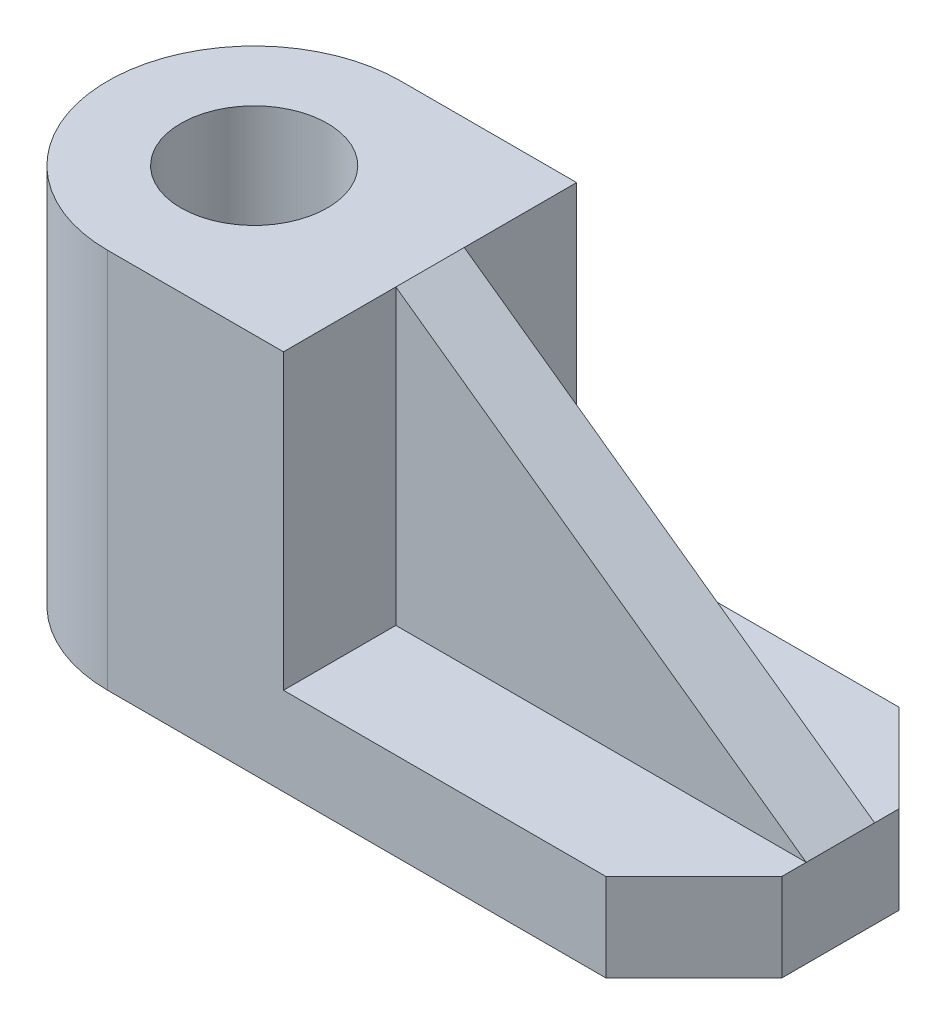
ISO-10303-21;
HEADER;
FILE_DESCRIPTION(('STEP AP214'),'2;1');
FILE_NAME('part.step','',(''),(''),'','','');
FILE_SCHEMA(('AUTOMOTIVE_DESIGN { 1 0 10303 214 1 1 1 1 }'));
ENDSEC;
DATA;
#1=APPLICATION_CONTEXT('core data for automotive mechanical design processes');
#2=APPLICATION_PROTOCOL_DEFINITION('international standard','automotive_design',2000,#1);
#3=PRODUCT_CONTEXT('',#1,'mechanical');
#4=PRODUCT('Part','Part','',(#3));
#5=PRODUCT_RELATED_PRODUCT_CATEGORY('part','',(#4));
#6=PRODUCT_DEFINITION_FORMATION('','',#4);
#7=PRODUCT_DEFINITION_CONTEXT('part definition',#1,'design');
#8=PRODUCT_DEFINITION('design','',#6,#7);
#9=PRODUCT_DEFINITION_SHAPE('','',#8);
#10=(LENGTH_UNIT() NAMED_UNIT(*) SI_UNIT(.MILLI.,.METRE.));
#11=(NAMED_UNIT(*) PLANE_ANGLE_UNIT() SI_UNIT($,.RADIAN.));
#12=(NAMED_UNIT(*) SI_UNIT($,.STERADIAN.) SOLID_ANGLE_UNIT());
#13=UNCERTAINTY_MEASURE_WITH_UNIT(LENGTH_MEASURE(1.E-05),#10,'distance_accuracy_value','');
#14=(GEOMETRIC_REPRESENTATION_CONTEXT(3) GLOBAL_UNCERTAINTY_ASSIGNED_CONTEXT((#13)) GLOBAL_UNIT_ASSIGNED_CONTEXT((#10,
#11,#12)) REPRESENTATION_CONTEXT('',''));
#15=CARTESIAN_POINT('',(0.,0.,0.));
#16=DIRECTION('',(0.,0.,1.));
#17=DIRECTION('',(1.,0.,0.));
#18=AXIS2_PLACEMENT_3D('',#15,#16,#17);
#19=CARTESIAN_POINT('',(0.,9.,0.));
#20=DIRECTION('',(0.,1.,0.));
#21=DIRECTION('',(0.,0.,1.));
#22=AXIS2_PLACEMENT_3D('',#19,#20,#21);
#23=PLANE('',#22);
#24=DIRECTION('',(0.,0.,1.));
#25=VECTOR('',#24,1.);
#26=CARTESIAN_POINT('',(-4.5,9.,0.));
#27=LINE('',#26,#25);
#28=CARTESIAN_POINT('',(-4.5,9.,-15.));
#29=VERTEX_POINT('',#28);
#30=CARTESIAN_POINT('',(-4.5,9.,-3.5));
#31=VERTEX_POINT('',#30);
#32=EDGE_CURVE('E166',#29,#31,#27,.T.);
#33=ORIENTED_EDGE('',*,*,#32,.T.);
#34=DIRECTION('',(1.,0.,0.));
#35=VECTOR('',#34,1.);
#36=CARTESIAN_POINT('',(37.5,9.,-3.5));
#37=LINE('',#36,#35);
#38=CARTESIAN_POINT('',(37.5,9.,-3.5));
#39=VERTEX_POINT('',#38);
#40=EDGE_CURVE('E59',#31,#39,#37,.T.);
#41=ORIENTED_EDGE('',*,*,#40,.T.);
#42=DIRECTION('',(0.,0.,-1.));
#43=VECTOR('',#42,1.);
#44=CARTESIAN_POINT('',(37.5,9.,-6.));
#45=LINE('',#44,#43);
#46=CARTESIAN_POINT('',(37.5,9.,-6.));
#47=VERTEX_POINT('',#46);
#48=EDGE_CURVE('E194',#39,#47,#45,.T.);
#49=ORIENTED_EDGE('',*,*,#48,.T.);
#50=DIRECTION('',(-0.707106781186548,0.,-0.707106781186547));
#51=VECTOR('',#50,1.);
#52=CARTESIAN_POINT('',(28.5,9.,-15.));
#53=LINE('',#52,#51);
#54=CARTESIAN_POINT('',(28.5,9.,-15.));
#55=VERTEX_POINT('',#54);
#56=EDGE_CURVE('E197',#47,#55,#53,.T.);
#57=ORIENTED_EDGE('',*,*,#56,.T.);
#58=DIRECTION('',(-1.,0.,0.));
#59=VECTOR('',#58,1.);
#60=CARTESIAN_POINT('',(-37.5,9.,-15.));
#61=LINE('',#60,#59);
#62=EDGE_CURVE('E200',#55,#29,#61,.T.);
#63=ORIENTED_EDGE('',*,*,#62,.T.);
#64=EDGE_LOOP('',(#33,#41,#49,#57,#63));
#65=FACE_BOUND('',#64,.T.);
#66=ADVANCED_FACE('F43',(#65),#23,.T.);
#67=CARTESIAN_POINT('',(-4.5,39.,0.));
#68=DIRECTION('',(1.,0.,0.));
#69=DIRECTION('',(0.,0.,-1.));
#70=AXIS2_PLACEMENT_3D('',#67,#68,#69);
#71=PLANE('',#70);
#72=DIRECTION('',(0.,0.,1.));
#73=VECTOR('',#72,1.);
#74=CARTESIAN_POINT('',(-4.5,39.,0.));
#75=LINE('',#74,#73);
#76=CARTESIAN_POINT('',(-4.5,39.,-15.));
#77=VERTEX_POINT('',#76);
#78=CARTESIAN_POINT('',(-4.5,39.,-3.5));
#79=VERTEX_POINT('',#78);
#80=EDGE_CURVE('E137',#77,#79,#75,.T.);
#81=ORIENTED_EDGE('',*,*,#80,.T.);
#82=DIRECTION('',(0.,-1.,0.));
#83=VECTOR('',#82,1.);
#84=CARTESIAN_POINT('',(-4.5,9.,-3.5));
#85=LINE('',#84,#83);
#86=EDGE_CURVE('E238',#79,#31,#85,.T.);
#87=ORIENTED_EDGE('',*,*,#86,.T.);
#88=ORIENTED_EDGE('',*,*,#32,.F.);
#89=DIRECTION('',(0.,-1.,0.));
#90=VECTOR('',#89,1.);
#91=CARTESIAN_POINT('',(-4.5,39.,-15.));
#92=LINE('',#91,#90);
#93=EDGE_CURVE('E177',#77,#29,#92,.T.);
#94=ORIENTED_EDGE('',*,*,#93,.F.);
#95=EDGE_LOOP('',(#81,#87,#88,#94));
#96=FACE_BOUND('',#95,.T.);
#97=ADVANCED_FACE('F265',(#96),#71,.T.);
#98=DIRECTION('',(1.,0.,0.));
#99=VECTOR('',#98,1.);
#100=CARTESIAN_POINT('',(37.5,9.,3.5));
#101=LINE('',#100,#99);
#102=CARTESIAN_POINT('',(-4.5,9.,3.5));
#103=VERTEX_POINT('',#102);
#104=CARTESIAN_POINT('',(37.5,9.,3.5));
#105=VERTEX_POINT('',#104);
#106=EDGE_CURVE('E151',#103,#105,#101,.T.);
#107=ORIENTED_EDGE('',*,*,#106,.F.);
#108=CARTESIAN_POINT('',(-4.5,9.,15.));
#109=VERTEX_POINT('',#108);
#110=EDGE_CURVE('E146',#103,#109,#27,.T.);
#111=ORIENTED_EDGE('',*,*,#110,.T.);
#112=DIRECTION('',(1.,0.,0.));
#113=VECTOR('',#112,1.);
#114=CARTESIAN_POINT('',(-37.5,9.,15.));
#115=LINE('',#114,#113);
#116=CARTESIAN_POINT('',(28.5,9.,15.));
#117=VERTEX_POINT('',#116);
#118=EDGE_CURVE('E186',#109,#117,#115,.T.);
#119=ORIENTED_EDGE('',*,*,#118,.T.);
#120=DIRECTION('',(0.707106781186548,0.,-0.707106781186547));
#121=VECTOR('',#120,1.);
#122=CARTESIAN_POINT('',(37.5,9.,6.));
#123=LINE('',#122,#121);
#124=CARTESIAN_POINT('',(37.5,9.,6.));
#125=VERTEX_POINT('',#124);
#126=EDGE_CURVE('E193',#117,#125,#123,.T.);
#127=ORIENTED_EDGE('',*,*,#126,.T.);
#128=EDGE_CURVE('E192',#125,#105,#45,.T.);
#129=ORIENTED_EDGE('',*,*,#128,.T.);
#130=EDGE_LOOP('',(#107,#111,#119,#127,#129));
#131=FACE_BOUND('',#130,.T.);
#132=ADVANCED_FACE('F266',(#131),#23,.T.);
#133=CARTESIAN_POINT('',(0.,0.,0.));
#134=DIRECTION('',(0.,1.,0.));
#135=DIRECTION('',(0.,0.,1.));
#136=AXIS2_PLACEMENT_3D('',#133,#134,#135);
#137=PLANE('',#136);
#138=CARTESIAN_POINT('',(-22.5,0.,0.));
#139=DIRECTION('',(0.,1.,0.));
#140=DIRECTION('',(0.,0.,1.));
#141=AXIS2_PLACEMENT_3D('',#138,#139,#140);
#142=CIRCLE('',#141,7.5);
#143=CARTESIAN_POINT('',(-22.5,0.,7.5));
#144=VERTEX_POINT('',#143);
#145=EDGE_CURVE('E242',#144,#144,#142,.T.);
#146=ORIENTED_EDGE('',*,*,#145,.T.);
#147=EDGE_LOOP('',(#146));
#148=FACE_BOUND('',#147,.T.);
#149=CARTESIAN_POINT('',(-22.5,0.,0.));
#150=DIRECTION('',(0.,1.,0.));
#151=DIRECTION('',(0.,0.,1.));
#152=AXIS2_PLACEMENT_3D('',#149,#150,#151);
#153=CIRCLE('',#152,15.);
#154=CARTESIAN_POINT('',(-22.5,0.,-15.));
#155=VERTEX_POINT('',#154);
#156=CARTESIAN_POINT('',(-22.5,0.,15.));
#157=VERTEX_POINT('',#156);
#158=EDGE_CURVE('E184',#155,#157,#153,.T.);
#159=ORIENTED_EDGE('',*,*,#158,.F.);
#160=DIRECTION('',(-1.,0.,0.));
#161=VECTOR('',#160,1.);
#162=CARTESIAN_POINT('',(-37.5,0.,-15.));
#163=LINE('',#162,#161);
#164=CARTESIAN_POINT('',(28.5,0.,-15.));
#165=VERTEX_POINT('',#164);
#166=EDGE_CURVE('E195',#165,#155,#163,.T.);
#167=ORIENTED_EDGE('',*,*,#166,.F.);
#168=DIRECTION('',(-0.707106781186548,0.,-0.707106781186547));
#169=VECTOR('',#168,1.);
#170=CARTESIAN_POINT('',(28.5,0.,-15.));
#171=LINE('',#170,#169);
#172=CARTESIAN_POINT('',(37.5,0.,-6.));
#173=VERTEX_POINT('',#172);
#174=EDGE_CURVE('E208',#173,#165,#171,.T.);
#175=ORIENTED_EDGE('',*,*,#174,.F.);
#176=DIRECTION('',(0.,0.,-1.));
#177=VECTOR('',#176,1.);
#178=CARTESIAN_POINT('',(37.5,0.,-6.));
#179=LINE('',#178,#177);
#180=CARTESIAN_POINT('',(37.5,0.,6.));
#181=VERTEX_POINT('',#180);
#182=EDGE_CURVE('E206',#181,#173,#179,.T.);
#183=ORIENTED_EDGE('',*,*,#182,.F.);
#184=DIRECTION('',(0.707106781186548,0.,-0.707106781186547));
#185=VECTOR('',#184,1.);
#186=CARTESIAN_POINT('',(37.5,0.,6.));
#187=LINE('',#186,#185);
#188=CARTESIAN_POINT('',(28.5,0.,15.));
#189=VERTEX_POINT('',#188);
#190=EDGE_CURVE('E204',#189,#181,#187,.T.);
#191=ORIENTED_EDGE('',*,*,#190,.F.);
#192=DIRECTION('',(1.,0.,0.));
#193=VECTOR('',#192,1.);
#194=CARTESIAN_POINT('',(-37.5,0.,15.));
#195=LINE('',#194,#193);
#196=EDGE_CURVE('E190',#157,#189,#195,.T.);
#197=ORIENTED_EDGE('',*,*,#196,.F.);
#198=EDGE_LOOP('',(#159,#167,#175,#183,#191,#197));
#199=FACE_BOUND('',#198,.T.);
#200=ADVANCED_FACE('F227',(#148,#199),#137,.F.);
#201=CARTESIAN_POINT('',(-37.5,9.,15.));
#202=DIRECTION('',(0.,0.,-1.));
#203=DIRECTION('',(-1.,0.,0.));
#204=AXIS2_PLACEMENT_3D('',#201,#202,#203);
#205=PLANE('',#204);
#206=DIRECTION('',(0.,1.,0.));
#207=VECTOR('',#206,1.);
#208=CARTESIAN_POINT('',(-22.5,0.,15.));
#209=LINE('',#208,#207);
#210=CARTESIAN_POINT('',(-22.5,39.,15.));
#211=VERTEX_POINT('',#210);
#212=EDGE_CURVE('E187',#157,#211,#209,.T.);
#213=ORIENTED_EDGE('',*,*,#212,.F.);
#214=ORIENTED_EDGE('',*,*,#196,.T.);
#215=DIRECTION('',(0.,-1.,0.));
#216=VECTOR('',#215,1.);
#217=CARTESIAN_POINT('',(28.5,9.,15.));
#218=LINE('',#217,#216);
#219=EDGE_CURVE('E11',#117,#189,#218,.T.);
#220=ORIENTED_EDGE('',*,*,#219,.F.);
#221=ORIENTED_EDGE('',*,*,#118,.F.);
#222=DIRECTION('',(0.,-1.,0.));
#223=VECTOR('',#222,1.);
#224=CARTESIAN_POINT('',(-4.5,39.,15.));
#225=LINE('',#224,#223);
#226=CARTESIAN_POINT('',(-4.5,39.,15.));
#227=VERTEX_POINT('',#226);
#228=EDGE_CURVE('E180',#227,#109,#225,.T.);
#229=ORIENTED_EDGE('',*,*,#228,.F.);
#230=DIRECTION('',(1.,0.,0.));
#231=VECTOR('',#230,1.);
#232=CARTESIAN_POINT('',(0.,39.,15.));
#233=LINE('',#232,#231);
#234=EDGE_CURVE('E138',#211,#227,#233,.T.);
#235=ORIENTED_EDGE('',*,*,#234,.F.);
#236=EDGE_LOOP('',(#213,#214,#220,#221,#229,#235));
#237=FACE_BOUND('',#236,.T.);
#238=ADVANCED_FACE('F44',(#237),#205,.F.);
#239=CARTESIAN_POINT('',(37.5,9.,6.));
#240=DIRECTION('',(-0.707106781186547,0.,-0.707106781186548));
#241=DIRECTION('',(-0.707106781186548,0.,0.707106781186547));
#242=AXIS2_PLACEMENT_3D('',#239,#240,#241);
#243=PLANE('',#242);
#244=ORIENTED_EDGE('',*,*,#190,.T.);
#245=DIRECTION('',(0.,-1.,0.));
#246=VECTOR('',#245,1.);
#247=CARTESIAN_POINT('',(37.5,9.,6.));
#248=LINE('',#247,#246);
#249=EDGE_CURVE('E51',#125,#181,#248,.T.);
#250=ORIENTED_EDGE('',*,*,#249,.F.);
#251=ORIENTED_EDGE('',*,*,#126,.F.);
#252=ORIENTED_EDGE('',*,*,#219,.T.);
#253=EDGE_LOOP('',(#244,#250,#251,#252));
#254=FACE_BOUND('',#253,.T.);
#255=ADVANCED_FACE('F278',(#254),#243,.F.);
#256=CARTESIAN_POINT('',(37.5,9.,-6.));
#257=DIRECTION('',(-1.,0.,0.));
#258=DIRECTION('',(0.,0.,1.));
#259=AXIS2_PLACEMENT_3D('',#256,#257,#258);
#260=PLANE('',#259);
#261=ORIENTED_EDGE('',*,*,#182,.T.);
#262=DIRECTION('',(0.,-1.,0.));
#263=VECTOR('',#262,1.);
#264=CARTESIAN_POINT('',(37.5,9.,-6.));
#265=LINE('',#264,#263);
#266=EDGE_CURVE('E212',#47,#173,#265,.T.);
#267=ORIENTED_EDGE('',*,*,#266,.F.);
#268=ORIENTED_EDGE('',*,*,#48,.F.);
#269=DIRECTION('',(0.,0.,-1.));
#270=VECTOR('',#269,1.);
#271=CARTESIAN_POINT('',(37.5,9.,3.5));
#272=LINE('',#271,#270);
#273=EDGE_CURVE('E63',#105,#39,#272,.T.);
#274=ORIENTED_EDGE('',*,*,#273,.F.);
#275=ORIENTED_EDGE('',*,*,#128,.F.);
#276=ORIENTED_EDGE('',*,*,#249,.T.);
#277=EDGE_LOOP('',(#261,#267,#268,#274,#275,#276));
#278=FACE_BOUND('',#277,.T.);
#279=ADVANCED_FACE('F218',(#278),#260,.F.);
#280=CARTESIAN_POINT('',(28.5,9.,-15.));
#281=DIRECTION('',(-0.707106781186547,0.,0.707106781186548));
#282=DIRECTION('',(0.707106781186548,0.,0.707106781186547));
#283=AXIS2_PLACEMENT_3D('',#280,#281,#282);
#284=PLANE('',#283);
#285=ORIENTED_EDGE('',*,*,#174,.T.);
#286=DIRECTION('',(0.,-1.,0.));
#287=VECTOR('',#286,1.);
#288=CARTESIAN_POINT('',(28.5,9.,-15.));
#289=LINE('',#288,#287);
#290=EDGE_CURVE('E205',#55,#165,#289,.T.);
#291=ORIENTED_EDGE('',*,*,#290,.F.);
#292=ORIENTED_EDGE('',*,*,#56,.F.);
#293=ORIENTED_EDGE('',*,*,#266,.T.);
#294=EDGE_LOOP('',(#285,#291,#292,#293));
#295=FACE_BOUND('',#294,.T.);
#296=ADVANCED_FACE('F233',(#295),#284,.F.);
#297=CARTESIAN_POINT('',(-37.5,9.,-15.));
#298=DIRECTION('',(0.,0.,1.));
#299=DIRECTION('',(1.,0.,0.));
#300=AXIS2_PLACEMENT_3D('',#297,#298,#299);
#301=PLANE('',#300);
#302=ORIENTED_EDGE('',*,*,#166,.T.);
#303=DIRECTION('',(0.,1.,0.));
#304=VECTOR('',#303,1.);
#305=CARTESIAN_POINT('',(-22.5,0.,-15.));
#306=LINE('',#305,#304);
#307=CARTESIAN_POINT('',(-22.5,39.,-15.));
#308=VERTEX_POINT('',#307);
#309=EDGE_CURVE('E185',#155,#308,#306,.T.);
#310=ORIENTED_EDGE('',*,*,#309,.T.);
#311=DIRECTION('',(-1.,0.,0.));
#312=VECTOR('',#311,1.);
#313=CARTESIAN_POINT('',(0.,39.,-15.));
#314=LINE('',#313,#312);
#315=EDGE_CURVE('E172',#77,#308,#314,.T.);
#316=ORIENTED_EDGE('',*,*,#315,.F.);
#317=ORIENTED_EDGE('',*,*,#93,.T.);
#318=ORIENTED_EDGE('',*,*,#62,.F.);
#319=ORIENTED_EDGE('',*,*,#290,.T.);
#320=EDGE_LOOP('',(#302,#310,#316,#317,#318,#319));
#321=FACE_BOUND('',#320,.T.);
#322=ADVANCED_FACE('F232',(#321),#301,.F.);
#323=CARTESIAN_POINT('',(-22.5,0.,0.));
#324=DIRECTION('',(0.,1.,0.));
#325=DIRECTION('',(0.,0.,1.));
#326=AXIS2_PLACEMENT_3D('',#323,#324,#325);
#327=CYLINDRICAL_SURFACE('',#326,15.);
#328=ORIENTED_EDGE('',*,*,#212,.T.);
#329=CARTESIAN_POINT('',(-22.5,39.,0.));
#330=DIRECTION('',(0.,1.,0.));
#331=DIRECTION('',(0.,0.,1.));
#332=AXIS2_PLACEMENT_3D('',#329,#330,#331);
#333=CIRCLE('',#332,15.);
#334=EDGE_CURVE('E171',#308,#211,#333,.T.);
#335=ORIENTED_EDGE('',*,*,#334,.F.);
#336=ORIENTED_EDGE('',*,*,#309,.F.);
#337=ORIENTED_EDGE('',*,*,#158,.T.);
#338=EDGE_LOOP('',(#328,#335,#336,#337));
#339=FACE_BOUND('',#338,.T.);
#340=ADVANCED_FACE('F257',(#339),#327,.T.);
#341=DIRECTION('',(0.,-1.,0.));
#342=VECTOR('',#341,1.);
#343=CARTESIAN_POINT('',(-4.5,9.,3.5));
#344=LINE('',#343,#342);
#345=CARTESIAN_POINT('',(-4.5,39.,3.5));
#346=VERTEX_POINT('',#345);
#347=EDGE_CURVE('E144',#346,#103,#344,.T.);
#348=ORIENTED_EDGE('',*,*,#347,.F.);
#349=EDGE_CURVE('E130',#346,#227,#75,.T.);
#350=ORIENTED_EDGE('',*,*,#349,.T.);
#351=ORIENTED_EDGE('',*,*,#228,.T.);
#352=ORIENTED_EDGE('',*,*,#110,.F.);
#353=EDGE_LOOP('',(#348,#350,#351,#352));
#354=FACE_BOUND('',#353,.T.);
#355=ADVANCED_FACE('F150',(#354),#71,.T.);
#356=CARTESIAN_POINT('',(-22.5,39.,0.));
#357=DIRECTION('',(0.,-1.,0.));
#358=DIRECTION('',(0.,0.,-1.));
#359=AXIS2_PLACEMENT_3D('',#356,#357,#358);
#360=CYLINDRICAL_SURFACE('',#359,7.5);
#361=CARTESIAN_POINT('',(-22.5,39.,0.));
#362=DIRECTION('',(0.,1.,0.));
#363=DIRECTION('',(0.,0.,1.));
#364=AXIS2_PLACEMENT_3D('',#361,#362,#363);
#365=CIRCLE('',#364,7.5);
#366=CARTESIAN_POINT('',(-22.5,39.,7.5));
#367=VERTEX_POINT('',#366);
#368=EDGE_CURVE('E143',#367,#367,#365,.T.);
#369=ORIENTED_EDGE('',*,*,#368,.T.);
#370=EDGE_LOOP('',(#369));
#371=FACE_BOUND('',#370,.T.);
#372=ORIENTED_EDGE('',*,*,#145,.F.);
#373=EDGE_LOOP('',(#372));
#374=FACE_BOUND('',#373,.T.);
#375=ADVANCED_FACE('F249',(#371,#374),#360,.F.);
#376=CARTESIAN_POINT('',(0.,39.,0.));
#377=DIRECTION('',(0.,1.,0.));
#378=DIRECTION('',(0.,0.,1.));
#379=AXIS2_PLACEMENT_3D('',#376,#377,#378);
#380=PLANE('',#379);
#381=ORIENTED_EDGE('',*,*,#368,.F.);
#382=EDGE_LOOP('',(#381));
#383=FACE_BOUND('',#382,.T.);
#384=ORIENTED_EDGE('',*,*,#80,.F.);
#385=ORIENTED_EDGE('',*,*,#315,.T.);
#386=ORIENTED_EDGE('',*,*,#334,.T.);
#387=ORIENTED_EDGE('',*,*,#234,.T.);
#388=ORIENTED_EDGE('',*,*,#349,.F.);
#389=DIRECTION('',(0.,0.,-1.));
#390=VECTOR('',#389,1.);
#391=CARTESIAN_POINT('',(-4.5,39.,3.5));
#392=LINE('',#391,#390);
#393=EDGE_CURVE('E134',#346,#79,#392,.T.);
#394=ORIENTED_EDGE('',*,*,#393,.T.);
#395=EDGE_LOOP('',(#384,#385,#386,#387,#388,#394));
#396=FACE_BOUND('',#395,.T.);
#397=ADVANCED_FACE('F128',(#383,#396),#380,.T.);
#398=CARTESIAN_POINT('',(-4.5,39.,3.5));
#399=DIRECTION('',(-0.581238193719096,-0.813733471206735,0.));
#400=DIRECTION('',(0.813733471206735,-0.581238193719096,0.));
#401=AXIS2_PLACEMENT_3D('',#398,#399,#400);
#402=PLANE('',#401);
#403=DIRECTION('',(-0.813733471206735,0.581238193719096,0.));
#404=VECTOR('',#403,1.);
#405=CARTESIAN_POINT('',(-4.5,39.,-3.5));
#406=LINE('',#405,#404);
#407=EDGE_CURVE('E155',#39,#79,#406,.T.);
#408=ORIENTED_EDGE('',*,*,#407,.T.);
#409=ORIENTED_EDGE('',*,*,#393,.F.);
#410=DIRECTION('',(-0.813733471206735,0.581238193719096,0.));
#411=VECTOR('',#410,1.);
#412=CARTESIAN_POINT('',(-4.5,39.,3.5));
#413=LINE('',#412,#411);
#414=EDGE_CURVE('E154',#105,#346,#413,.T.);
#415=ORIENTED_EDGE('',*,*,#414,.F.);
#416=ORIENTED_EDGE('',*,*,#273,.T.);
#417=EDGE_LOOP('',(#408,#409,#415,#416));
#418=FACE_BOUND('',#417,.T.);
#419=ADVANCED_FACE('F159',(#418),#402,.F.);
#420=CARTESIAN_POINT('',(0.,0.,3.5));
#421=DIRECTION('',(0.,0.,1.));
#422=DIRECTION('',(1.,0.,0.));
#423=AXIS2_PLACEMENT_3D('',#420,#421,#422);
#424=PLANE('',#423);
#425=ORIENTED_EDGE('',*,*,#347,.T.);
#426=ORIENTED_EDGE('',*,*,#106,.T.);
#427=ORIENTED_EDGE('',*,*,#414,.T.);
#428=EDGE_LOOP('',(#425,#426,#427));
#429=FACE_BOUND('',#428,.T.);
#430=ADVANCED_FACE('F156',(#429),#424,.T.);
#431=CARTESIAN_POINT('',(0.,0.,-3.5));
#432=DIRECTION('',(0.,0.,1.));
#433=DIRECTION('',(1.,0.,0.));
#434=AXIS2_PLACEMENT_3D('',#431,#432,#433);
#435=PLANE('',#434);
#436=ORIENTED_EDGE('',*,*,#86,.F.);
#437=ORIENTED_EDGE('',*,*,#407,.F.);
#438=ORIENTED_EDGE('',*,*,#40,.F.);
#439=EDGE_LOOP('',(#436,#437,#438));
#440=FACE_BOUND('',#439,.T.);
#441=ADVANCED_FACE('F239',(#440),#435,.F.);
#442=CLOSED_SHELL('',(#66,#97,#132,#200,#238,#255,#279,#296,#322,#340,#355,#375,#397,#419,#430,#441));
#443=MANIFOLD_SOLID_BREP('B2',#442);
#444=ADVANCED_BREP_SHAPE_REPRESENTATION('',(#18,#443),#14);
#445=SHAPE_DEFINITION_REPRESENTATION(#9,#444);
ENDSEC;
END-ISO-10303-21;
